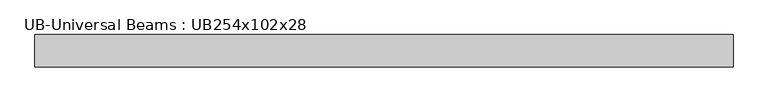
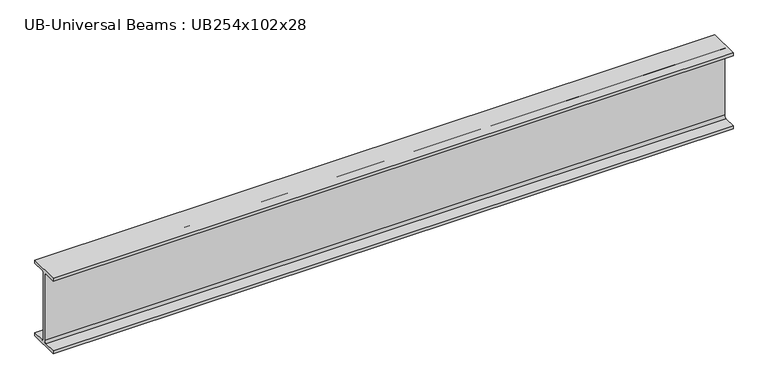
"""IFC4 building model written with IfcOpenShell, lengths in millimetres: beam geometry, UB-Universal Beams : UB254x102x28."""

from ifc_helpers import new_model, si_unit, point, frame, frame_2d, origin, place, context, project, spatial, polyline, circle_curve, trimmed, segment, composite_curve, outline, extrude, source, transform, mapped, element, save


def ub_universal_beams_ub254x102x28_1ec9d6d8(model_context):
    return source(origin(), model_context, "Body", "SweptSolid", [
        extrude(outline(composite_curve([segment(polyline([(51.1, -120.2), (51.1, -130.2), (-51.1, -130.2), (-51.1, -120.2), (-10.75, -120.2)]), True, "CONTINUOUS"), segment(trimmed(circle_curve(frame_2d((-10.75, -112.6)), 7.6), [point((-10.75, -120.2))], [point((-3.15, -112.6))], True, "CARTESIAN"), True, "CONTINUOUS"), segment(polyline([(-3.15, -112.6), (-3.15, 112.6)]), True, "CONTINUOUS"), segment(trimmed(circle_curve(frame_2d((-10.75, 112.6)), 7.6), [point((-3.15, 112.6))], [point((-10.75, 120.2))], True, "CARTESIAN"), True, "CONTINUOUS"), segment(polyline([(-10.75, 120.2), (-51.1, 120.2), (-51.1, 130.2), (51.1, 130.2), (51.1, 120.2), (10.75, 120.2)]), True, "CONTINUOUS"), segment(trimmed(circle_curve(frame_2d((10.75, 112.6)), 7.6), [point((10.75, 120.2))], [point((3.15, 112.6))], True, "CARTESIAN"), True, "CONTINUOUS"), segment(polyline([(3.15, 112.6), (3.15, -112.6)]), True, "CONTINUOUS"), segment(trimmed(circle_curve(frame_2d((10.75, -112.6)), 7.6), [point((3.15, -112.6))], [point((10.75, -120.2))], True, "CARTESIAN"), True, "CONTINUOUS"), segment(polyline([(10.75, -120.2), (51.1, -120.2)]), True, "CONTINUOUS")], self_intersect=False)), frame((-1044.15, 0.0, 0.0), z_axis=(1.0, 0.0, 0.0), x_axis=(0.0, 1.0, 0.0)), (0.0, 0.0, 1.0), 2215.4),
    ])


if __name__ == "__main__":
    model = new_model("IFC4")
    model_context = context("Model", 3, world=origin())
    ifc_project = project(units=[si_unit("LENGTHUNIT", "METRE", prefix="MILLI")], contexts=[model_context])
    site = spatial("IfcSite", under=ifc_project)
    building = spatial("IfcBuilding", under=site)
    placement = place(None, origin())
    ub_universal_beams_ub254x102x28_shape = ub_universal_beams_ub254x102x28_1ec9d6d8(model_context)
    element("IfcBeam", 1, ObjectType="UB-Universal Beams : UB254x102x28", at=placement, inside=building, context=model_context, shape_type="MappedRepresentation", body=[
        mapped(ub_universal_beams_ub254x102x28_shape, transform((0.0, 0.0, 0.0), x_axis=(1.0, 0.0, 0.0), y_axis=(0.0, 1.0, 0.0), z_axis=(0.0, 0.0, 1.0))),
    ])
    save(model, "model.ifc")

# Revit data of these elements
# Type "UB-Universal Beams : UB254x102x28"
#   Section Name Key = "UB254X102X28"
#   Width = 10.22 cm
#   Web Thickness = 0.63 cm
#   Web Fillet = 0.76 cm
#   Warping Constant = 28000.0 cm⁶
#   Torsional Moment of Inertia = 9.57 cm⁴
#   Section Area = 36.1 cm²
#   Plastic Modulus weak axis = 54.8 cm³
#   Plastic Modulus strong axis = 353.0 cm³
#   Nominal Weight = 28.2999 kgf/m
#   Moment of Inertia weak axis = 179.00 cm⁴
#   Moment of Inertia strong axis = 4005.00 cm⁴
#   Height = 26.04 cm
#   Flange Thickness = 1.0 cm
#   Elastic Modulus weak axis = 34.9 cm³
#   Elastic Modulus strong axis = 308.0 cm³
#   Centroid Vertical = 13.02 cm
#   Centroid Horizontal = 5.11 cm
#   Bolt Spacing = 5.4 cm
#   Length [instance default] = 4' - 11.05512"
#   Structural Material [instance default] = Metal - Steel 43-275
#   Type Comments = ""
#   Assembly Code = ""
# Element 1 (IfcBeam, "UB-Universal Beams : UB254x102x28")
#   Materials on its faces: "Metal - Steel 43-275"
# Materials
#   "Metal - Steel 43-275": class "Metal", colour RGB 247 247 247, transparency 0, Cost = 0
